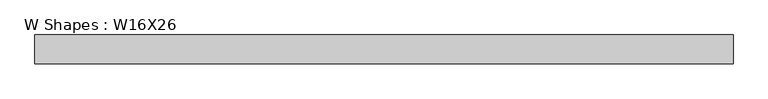
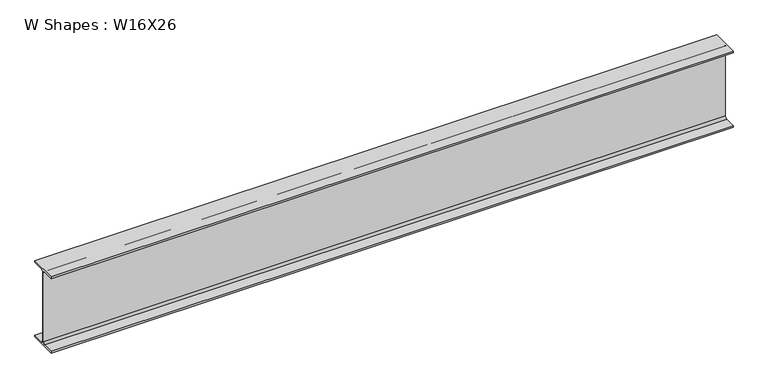
"""IFC4 building model written with IfcOpenShell, lengths in millimetres: beam geometry, W Shapes : W16X26."""

from ifc_helpers import new_model, si_unit, point, frame, frame_2d, origin, place, context, project, spatial, polyline, circle_curve, trimmed, segment, composite_curve, outline, extrude, source, transform, mapped, element, save


def w_shapes_w16x26_5730d789(model_context):
    return source(origin(), model_context, "Body", "SweptSolid", [
        extrude(outline(composite_curve([segment(polyline([(69.85, -190.627), (69.85, -199.39), (-69.85, -199.39), (-69.85, -190.627), (-13.3858, -190.627)]), True, "CONTINUOUS"), segment(trimmed(circle_curve(frame_2d((-13.3858, -180.4162)), 10.2108), [point((-13.3858, -190.627))], [point((-3.175, -180.4162))], True, "CARTESIAN"), True, "CONTINUOUS"), segment(polyline([(-3.175, -180.4162), (-3.175, 180.4162)]), True, "CONTINUOUS"), segment(trimmed(circle_curve(frame_2d((-13.3858, 180.4162)), 10.2108), [point((-3.175, 180.4162))], [point((-13.3858, 190.627))], True, "CARTESIAN"), True, "CONTINUOUS"), segment(polyline([(-13.3858, 190.627), (-69.85, 190.627), (-69.85, 199.39), (69.85, 199.39), (69.85, 190.627), (13.3858, 190.627)]), True, "CONTINUOUS"), segment(trimmed(circle_curve(frame_2d((13.3858, 180.4162)), 10.2108), [point((13.3858, 190.627))], [point((3.175, 180.4162))], True, "CARTESIAN"), True, "CONTINUOUS"), segment(polyline([(3.175, 180.4162), (3.175, -180.4162)]), True, "CONTINUOUS"), segment(trimmed(circle_curve(frame_2d((13.3858, -180.4162)), 10.2108), [point((3.175, -180.4162))], [point((13.3858, -190.627))], True, "CARTESIAN"), True, "CONTINUOUS"), segment(polyline([(13.3858, -190.627), (69.85, -190.627)]), True, "CONTINUOUS")], self_intersect=False)), frame((-1689.1, 0.0, 0.0), z_axis=(1.0, 0.0, 0.0), x_axis=(0.0, 1.0, 0.0)), (0.0, 0.0, 1.0), 3378.2),
    ])


if __name__ == "__main__":
    model = new_model("IFC4")
    model_context = context("Model", 3, world=origin())
    ifc_project = project(units=[si_unit("LENGTHUNIT", "METRE", prefix="MILLI")], contexts=[model_context])
    site = spatial("IfcSite", under=ifc_project)
    building = spatial("IfcBuilding", under=site)
    placement = place(None, origin())
    w_shapes_w16x26_shape = w_shapes_w16x26_5730d789(model_context)
    element("IfcBeam", 1, ObjectType="W Shapes : W16X26", at=placement, inside=building, context=model_context, shape_type="MappedRepresentation", body=[
        mapped(w_shapes_w16x26_shape, transform((0.0, 0.0, 0.0), x_axis=(1.0, 0.0, 0.0), y_axis=(0.0, 1.0, 0.0), z_axis=(0.0, 0.0, 1.0))),
    ])
    save(model, "model.ifc")

# Revit data of these elements
# Type "W Shapes : W16X26"
#   Section Name Key = "W16x26"
#   Assembly Code = "B10"
#   Width = 5.500"
#   Web Thickness = 0.250"
#   Web Fillet = 0.402"
#   Warping Constant = 565.00 in⁶
#   Torsional Moment of Inertia = 0.262 in⁴
#   Section Area = 7.68 in²
#   Plastic Modulus weak axis = 5.48 in³
#   Plastic Modulus strong axis = 44.20 in³
#   Perimeter = 52.20 ft²/ft
#   Nominal Weight = 26.00 lbf/ft
#   Moment of Inertia weak axis = 9.59 in⁴
#   Moment of Inertia strong axis = 301.00 in⁴
#   Height = 15.700"
#   Flange Thickness = 0.345"
#   Elastic Modulus weak axis = 3.49 in³
#   Elastic Modulus strong axis = 38.40 in³
#   Centroid Vertical = 7.850"
#   Centroid Horizontal = 2.750"
#   Bolt Spacing = 0' - 3 1/2"
#   Length [instance default] = 5' - 0"
#   Structural Material [instance default] = Steel ASTM A992
#   Principal Axes Angle = 0
# Element 1 (IfcBeam, "W Shapes : W16X26")
#   Materials on its faces: "Steel ASTM A992"
# Materials
#   "Steel ASTM A992": class "Metal", colour RGB 199 199 199, transparency 0, Description = "Structural steel 50ksi", Cost = 0
